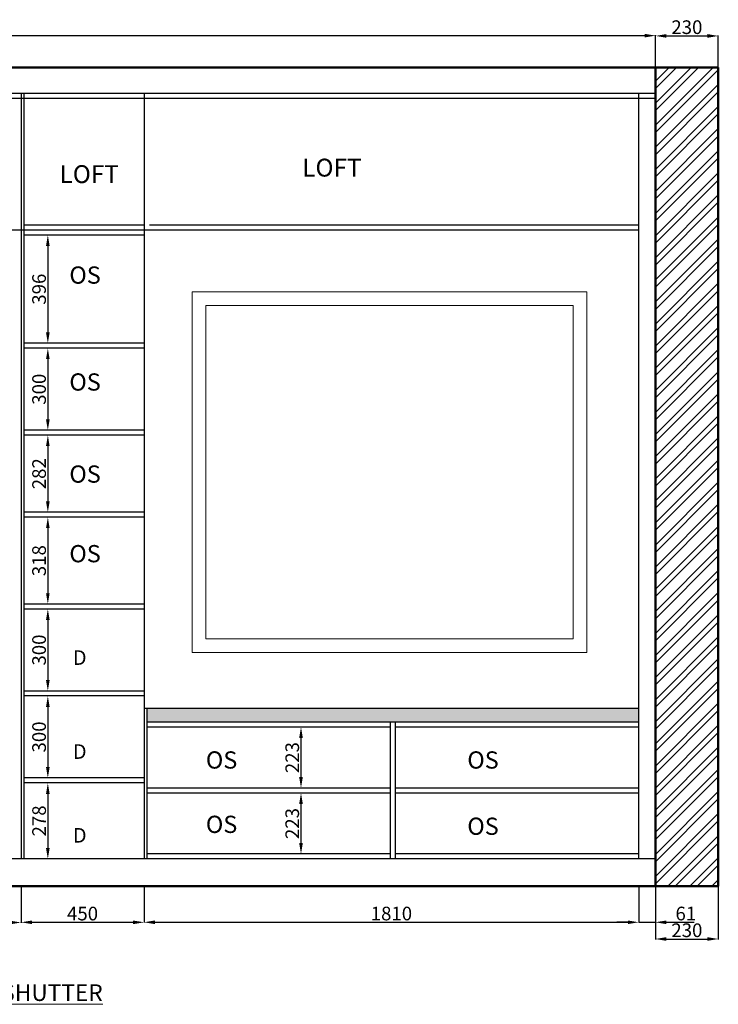
# Model space of a CAD drawing. Units: millimetres. Extents: x -513 to 5600, y -432 to 3172.
# Tile 2 of 2: x 3044 to 5600, y -432 to 3170. Entities that reach past the tile are written whole.
import ezdxf

# ---------------------------------------------------------------- set-up
doc = ezdxf.new("R2010")
doc.units = ezdxf.units.MM
for name, color, linetype, lineweight in [('A-ANNO-DIMS', 2, 'Continuous', 18), ('A-ANNO-TEXT', 7, 'Continuous', 18), ('A-ELEV-PATT', 8, 'Continuous', 13), ('A-FURN', 3, 'Continuous', 25), ('A-GLAZ', 4, 'Continuous', 18), ('A-WALL', 7, 'Continuous', 50), ('A-WALL-PATT', 8, 'Continuous', 13)]:
    doc.layers.add(name, color=color, linetype=linetype, lineweight=lineweight)
doc.styles.get("Standard").update_dxf_attribs({"font": 'arial.ttf'})
doc.dimstyles.new('ISO-25', dxfattribs={"dimtxt": 50, "dimasz": 40, "dimexe": 1.25, "dimexo": 0.625, "dimgap": 0, "dimtad": 1, "dimtxsty": 'Standard', "dimcen": 2.5, "dimclrt": 6, "dimadec": 0, "dimazin": 0, "dimtfac": 1, "dimtmove": 0, "dimatfit": 3, "dimfxl": 1, "dimarcsym": 0})

# ---------------------------------------------------------------- blocks, each defined once
blk = doc.blocks.new('*D11')
at = {"layer": 'A-ANNO-DIMS', "color": 0, "lineweight": -2, "transparency": 16777216}
for p, q in [((2129, -0.6), (2129, -133.8)), ((3049, -0.6), (3049, -133.8)), ((2169, -132.6), (3009, -132.6))]:
    blk.add_line(p, q, dxfattribs=at)
at = {"layer": 'A-ANNO-DIMS', "color": 0, "transparency": 16777216}
for points in [[(2169, -125.9), (2169, -139.2), (2129, -132.6)], [(3009, -125.9), (3009, -139.2), (3049, -132.6)]]:
    blk.add_solid(points, dxfattribs=at)
at = {"layer": 'Defpoints', "color": 0, "transparency": 16777216}
for p in [(2129, 0), (3049, 0), (3049, -132.6)]:
    blk.add_point(p, dxfattribs=at)
at = {"layer": 'A-ANNO-DIMS', "color": 0, "transparency": 16777216, "insert": (2589, -107), "char_height": 50, "attachment_point": 5}
blk.add_mtext('920', dxfattribs=at)
blk = doc.blocks.new('*D12')
at = {"layer": 'A-ANNO-DIMS', "color": 0, "lineweight": -2, "transparency": 16777216}
for p, q in [((3049, -0.6), (3049, -133.2)), ((3499, -0.6), (3499, -133.2)), ((3089, -131.9), (3459, -131.9))]:
    blk.add_line(p, q, dxfattribs=at)
at = {"layer": 'A-ANNO-DIMS', "color": 0, "transparency": 16777216}
for points in [[(3089, -125.3), (3089, -138.6), (3049, -131.9)], [(3459, -125.3), (3459, -138.6), (3499, -131.9)]]:
    blk.add_solid(points, dxfattribs=at)
at = {"layer": 'Defpoints', "color": 0, "transparency": 16777216}
for p in [(3049, 0), (3499, 0), (3499, -131.9)]:
    blk.add_point(p, dxfattribs=at)
at = {"layer": 'A-ANNO-DIMS', "color": 0, "transparency": 16777216, "insert": (3274, -106.4), "char_height": 50, "attachment_point": 5}
blk.add_mtext('450', dxfattribs=at)
blk = doc.blocks.new('*D13')
at = {"layer": 'A-ANNO-DIMS', "color": 0, "lineweight": -2, "transparency": 16777216}
for p, q in [((3499, -0.6), (3499, -133.1)), ((5309, -0.6), (5309, -133.1)), ((3539, -131.8), (5269, -131.8))]:
    blk.add_line(p, q, dxfattribs=at)
at = {"layer": 'A-ANNO-DIMS', "color": 0, "transparency": 16777216}
for points in [[(3539, -125.2), (3539, -138.5), (3499, -131.8)], [(5269, -125.2), (5269, -138.5), (5309, -131.8)]]:
    blk.add_solid(points, dxfattribs=at)
at = {"layer": 'Defpoints', "color": 0, "transparency": 16777216}
for p in [(3499, 0), (5309, 0), (5309, -131.8)]:
    blk.add_point(p, dxfattribs=at)
at = {"layer": 'A-ANNO-DIMS', "color": 0, "transparency": 16777216, "insert": (4404, -106.3), "char_height": 50, "attachment_point": 5}
blk.add_mtext('1810', dxfattribs=at)
blk = doc.blocks.new('*D14')
at = {"layer": 'A-ANNO-DIMS', "color": 0, "lineweight": -2, "transparency": 16777216}
for p, q in [((5309, -0.6), (5309, -133.1)), ((5370, -0.6), (5370, -133.1)), ((5269, -131.8), (5229, -131.8)), ((5309, -131.8), (5370, -131.8)), ((5410, -131.8), (5512.2, -131.8))]:
    blk.add_line(p, q, dxfattribs=at)
at = {"layer": 'A-ANNO-DIMS', "color": 0, "transparency": 16777216}
for points in [[(5269, -125.2), (5269, -138.5), (5309, -131.8)], [(5410, -125.2), (5410, -138.5), (5370, -131.8)]]:
    blk.add_solid(points, dxfattribs=at)
at = {"layer": 'Defpoints', "color": 0, "transparency": 16777216}
for p in [(5309, 0), (5370, 0), (5370, -131.8)]:
    blk.add_point(p, dxfattribs=at)
at = {"layer": 'A-ANNO-DIMS', "color": 0, "transparency": 16777216, "insert": (5481.1, -106.3), "char_height": 50, "attachment_point": 5}
blk.add_mtext('61', dxfattribs=at)
blk = doc.blocks.new('*D15')
at = {"layer": 'A-ANNO-DIMS', "color": 0, "lineweight": -2, "transparency": 16777216}
for p, q in [((5370, -0.6), (5370, -194.2)), ((5600, -0.6), (5600, -194.2)), ((5410, -193), (5560, -193))]:
    blk.add_line(p, q, dxfattribs=at)
at = {"layer": 'A-ANNO-DIMS', "color": 0, "transparency": 16777216}
for points in [[(5410, -186.3), (5410, -199.6), (5370, -193)], [(5560, -186.3), (5560, -199.6), (5600, -193)]]:
    blk.add_solid(points, dxfattribs=at)
at = {"layer": 'Defpoints', "color": 0, "transparency": 16777216}
for p in [(5370, 0), (5600, 0), (5600, -193)]:
    blk.add_point(p, dxfattribs=at)
at = {"layer": 'A-ANNO-DIMS', "color": 0, "transparency": 16777216, "insert": (5485, -167.4), "char_height": 50, "attachment_point": 5}
blk.add_mtext('230', dxfattribs=at)
blk = doc.blocks.new('*D30')
at = {"layer": 'A-ANNO-DIMS', "color": 0, "lineweight": -2, "transparency": 16777216}
for p, q in [((3147.6, 2382), (3148.2, 2382)), ((3147, 2342), (3147, 2026)), ((3147.6, 1986), (3148.2, 1986))]:
    blk.add_line(p, q, dxfattribs=at)
at = {"layer": 'A-ANNO-DIMS', "color": 0, "transparency": 16777216}
for points in [[(3140.3, 2342), (3153.6, 2342), (3147, 2382)], [(3140.3, 2026), (3153.6, 2026), (3147, 1986)]]:
    blk.add_solid(points, dxfattribs=at)
at = {"layer": 'Defpoints', "color": 0, "transparency": 16777216}
for p in [(3147, 2382), (3147, 1986), (3147, 1986)]:
    blk.add_point(p, dxfattribs=at)
at = {"layer": 'A-ANNO-DIMS', "color": 0, "transparency": 16777216, "insert": (3121.4, 2184), "char_height": 50, "attachment_point": 5, "rotation": 90}
blk.add_mtext('396', dxfattribs=at)
blk = doc.blocks.new('*D31')
at = {"layer": 'A-ANNO-DIMS', "color": 0, "lineweight": -2, "transparency": 16777216}
for p, q in [((3147.6, 1968), (3148.2, 1968)), ((3147, 1928), (3147, 1708)), ((3147.6, 1668), (3148.2, 1668))]:
    blk.add_line(p, q, dxfattribs=at)
at = {"layer": 'A-ANNO-DIMS', "color": 0, "transparency": 16777216}
for points in [[(3140.3, 1928), (3153.6, 1928), (3147, 1968)], [(3140.3, 1708), (3153.6, 1708), (3147, 1668)]]:
    blk.add_solid(points, dxfattribs=at)
at = {"layer": 'Defpoints', "color": 0, "transparency": 16777216}
for p in [(3147, 1968), (3147, 1668), (3147, 1668)]:
    blk.add_point(p, dxfattribs=at)
at = {"layer": 'A-ANNO-DIMS', "color": 0, "transparency": 16777216, "insert": (3121.4, 1818), "char_height": 50, "attachment_point": 5, "rotation": 90}
blk.add_mtext('300', dxfattribs=at)
blk = doc.blocks.new('*D32')
at = {"layer": 'A-ANNO-DIMS', "color": 0, "lineweight": -2, "transparency": 16777216}
for p, q in [((3147.6, 1650), (3148.2, 1650)), ((3147, 1610), (3147, 1408)), ((3147.6, 1368), (3148.2, 1368))]:
    blk.add_line(p, q, dxfattribs=at)
at = {"layer": 'A-ANNO-DIMS', "color": 0, "transparency": 16777216}
for points in [[(3140.3, 1610), (3153.6, 1610), (3147, 1650)], [(3140.3, 1408), (3153.6, 1408), (3147, 1368)]]:
    blk.add_solid(points, dxfattribs=at)
at = {"layer": 'Defpoints', "color": 0, "transparency": 16777216}
for p in [(3147, 1650), (3147, 1368), (3147, 1368)]:
    blk.add_point(p, dxfattribs=at)
at = {"layer": 'A-ANNO-DIMS', "color": 0, "transparency": 16777216, "insert": (3121.5, 1509), "char_height": 50, "attachment_point": 5, "rotation": 90}
blk.add_mtext('282', dxfattribs=at)
blk = doc.blocks.new('*D33')
at = {"layer": 'A-ANNO-DIMS', "color": 0, "lineweight": -2, "transparency": 16777216}
for p, q in [((3147.6, 1350), (3148.2, 1350)), ((3147, 1310), (3147, 1072)), ((3147.6, 1032), (3148.2, 1032))]:
    blk.add_line(p, q, dxfattribs=at)
at = {"layer": 'A-ANNO-DIMS', "color": 0, "transparency": 16777216}
for points in [[(3140.3, 1310), (3153.6, 1310), (3147, 1350)], [(3140.3, 1072), (3153.6, 1072), (3147, 1032)]]:
    blk.add_solid(points, dxfattribs=at)
at = {"layer": 'Defpoints', "color": 0, "transparency": 16777216}
for p in [(3147, 1350), (3147, 1032), (3147, 1032)]:
    blk.add_point(p, dxfattribs=at)
at = {"layer": 'A-ANNO-DIMS', "color": 0, "transparency": 16777216, "insert": (3121.4, 1191), "char_height": 50, "attachment_point": 5, "rotation": 90}
blk.add_mtext('318', dxfattribs=at)
blk = doc.blocks.new('*D34')
at = {"layer": 'A-ANNO-DIMS', "color": 0, "lineweight": -2, "transparency": 16777216}
for p, q in [((3147.6, 1014), (3148.2, 1014)), ((3147, 974), (3147, 754)), ((3147.6, 714), (3148.2, 714))]:
    blk.add_line(p, q, dxfattribs=at)
at = {"layer": 'A-ANNO-DIMS', "color": 0, "transparency": 16777216}
for points in [[(3140.3, 974), (3153.6, 974), (3147, 1014)], [(3140.3, 754), (3153.6, 754), (3147, 714)]]:
    blk.add_solid(points, dxfattribs=at)
at = {"layer": 'Defpoints', "color": 0, "transparency": 16777216}
for p in [(3147, 1014), (3147, 714), (3147, 714)]:
    blk.add_point(p, dxfattribs=at)
at = {"layer": 'A-ANNO-DIMS', "color": 0, "transparency": 16777216, "insert": (3121.4, 864), "char_height": 50, "attachment_point": 5, "rotation": 90}
blk.add_mtext('300', dxfattribs=at)
blk = doc.blocks.new('*D35')
at = {"layer": 'A-ANNO-DIMS', "color": 0, "lineweight": -2, "transparency": 16777216}
for p, q in [((3147.6, 696), (3148.2, 696)), ((3147, 656), (3147, 436)), ((3147.6, 396), (3148.2, 396))]:
    blk.add_line(p, q, dxfattribs=at)
at = {"layer": 'A-ANNO-DIMS', "color": 0, "transparency": 16777216}
for points in [[(3140.3, 656), (3153.6, 656), (3147, 696)], [(3140.3, 436), (3153.6, 436), (3147, 396)]]:
    blk.add_solid(points, dxfattribs=at)
at = {"layer": 'Defpoints', "color": 0, "transparency": 16777216}
for p in [(3147, 696), (3147, 396), (3147, 396)]:
    blk.add_point(p, dxfattribs=at)
at = {"layer": 'A-ANNO-DIMS', "color": 0, "transparency": 16777216, "insert": (3121.4, 546), "char_height": 50, "attachment_point": 5, "rotation": 90}
blk.add_mtext('300', dxfattribs=at)
blk = doc.blocks.new('*D36')
at = {"layer": 'A-ANNO-DIMS', "color": 0, "lineweight": -2, "transparency": 16777216}
for p, q in [((3147.6, 378), (3148.2, 378)), ((3147, 338), (3147, 140)), ((3147.6, 100), (3148.2, 100))]:
    blk.add_line(p, q, dxfattribs=at)
at = {"layer": 'A-ANNO-DIMS', "color": 0, "transparency": 16777216}
for points in [[(3140.3, 338), (3153.6, 338), (3147, 378)], [(3140.3, 140), (3153.6, 140), (3147, 100)]]:
    blk.add_solid(points, dxfattribs=at)
at = {"layer": 'Defpoints', "color": 0, "transparency": 16777216}
for p in [(3147, 378), (3147, 100), (3147, 100)]:
    blk.add_point(p, dxfattribs=at)
at = {"layer": 'A-ANNO-DIMS', "color": 0, "transparency": 16777216, "insert": (3121.5, 239), "char_height": 50, "attachment_point": 5, "rotation": 90}
blk.add_mtext('278', dxfattribs=at)
blk = doc.blocks.new('*D37')
at = {"layer": 'A-ANNO-DIMS', "color": 0, "lineweight": -2, "transparency": 16777216}
for p, q in [((4073.8, 582), (4074.4, 582)), ((4073.2, 542), (4073.2, 399)), ((4073.8, 359), (4074.4, 359))]:
    blk.add_line(p, q, dxfattribs=at)
at = {"layer": 'A-ANNO-DIMS', "color": 0, "transparency": 16777216}
for points in [[(4066.5, 542), (4079.9, 542), (4073.2, 582)], [(4066.5, 399), (4079.9, 399), (4073.2, 359)]]:
    blk.add_solid(points, dxfattribs=at)
at = {"layer": 'Defpoints', "color": 0, "transparency": 16777216}
for p in [(4073.2, 582), (4073.2, 359), (4073.2, 359)]:
    blk.add_point(p, dxfattribs=at)
at = {"layer": 'A-ANNO-DIMS', "color": 0, "transparency": 16777216, "insert": (4047.6, 470.5), "char_height": 50, "attachment_point": 5, "rotation": 90}
blk.add_mtext('223', dxfattribs=at)
blk = doc.blocks.new('*D38')
at = {"layer": 'A-ANNO-DIMS', "color": 0, "lineweight": -2, "transparency": 16777216}
for p, q in [((4073.8, 341), (4074.4, 341)), ((4073.2, 301), (4073.2, 158)), ((4073.8, 118), (4074.4, 118))]:
    blk.add_line(p, q, dxfattribs=at)
at = {"layer": 'A-ANNO-DIMS', "color": 0, "transparency": 16777216}
for points in [[(4066.5, 301), (4079.9, 301), (4073.2, 341)], [(4066.5, 158), (4079.9, 158), (4073.2, 118)]]:
    blk.add_solid(points, dxfattribs=at)
at = {"layer": 'Defpoints', "color": 0, "transparency": 16777216}
for p in [(4073.2, 341), (4073.2, 118), (4073.2, 118)]:
    blk.add_point(p, dxfattribs=at)
at = {"layer": 'A-ANNO-DIMS', "color": 0, "transparency": 16777216, "insert": (4047.6, 229.5), "char_height": 50, "attachment_point": 5, "rotation": 90}
blk.add_mtext('223', dxfattribs=at)
blk = doc.blocks.new('*D40')
at = {"layer": 'A-ANNO-DIMS', "color": 0, "lineweight": -2, "transparency": 16777216}
for p, q in [((230, 2995.6), (230, 3112.7)), ((270, 3111.4), (5330, 3111.4)), ((5370, 2995.6), (5370, 3112.7))]:
    blk.add_line(p, q, dxfattribs=at)
at = {"layer": 'A-ANNO-DIMS', "color": 0, "transparency": 16777216}
for points in [[(270, 3118.1), (270, 3104.8), (230, 3111.4)], [(5330, 3118.1), (5330, 3104.8), (5370, 3111.4)]]:
    blk.add_solid(points, dxfattribs=at)
at = {"layer": 'Defpoints', "color": 0, "transparency": 16777216}
for p in [(5370, 3111.4), (230, 2995), (5370, 2995)]:
    blk.add_point(p, dxfattribs=at)
at = {"layer": 'A-ANNO-DIMS', "color": 0, "transparency": 16777216, "insert": (2800, 3136.9), "char_height": 50, "attachment_point": 5}
blk.add_mtext('5140', dxfattribs=at)
blk = doc.blocks.new('*D41')
at = {"layer": 'A-ANNO-DIMS', "color": 0, "lineweight": -2, "transparency": 16777216}
for p, q in [((5370, 2995.6), (5370, 3111.6)), ((5410, 3110.4), (5560, 3110.4)), ((5600, 2995.6), (5600, 3111.6))]:
    blk.add_line(p, q, dxfattribs=at)
at = {"layer": 'A-ANNO-DIMS', "color": 0, "transparency": 16777216}
for points in [[(5410, 3117.1), (5410, 3103.7), (5370, 3110.4)], [(5560, 3117.1), (5560, 3103.7), (5600, 3110.4)]]:
    blk.add_solid(points, dxfattribs=at)
at = {"layer": 'Defpoints', "color": 0, "transparency": 16777216}
for p in [(5600, 3110.4), (5370, 2995), (5600, 2995)]:
    blk.add_point(p, dxfattribs=at)
at = {"layer": 'A-ANNO-DIMS', "color": 0, "transparency": 16777216, "insert": (5485, 3135.9), "char_height": 50, "attachment_point": 5}
blk.add_mtext('230', dxfattribs=at)

msp = doc.modelspace()

# ---------------------------------------------------------------- hatches: boundary and pattern name
at = {"layer": 'A-ELEV-PATT'}
h = msp.add_hatch(color=256, dxfattribs=at)
h.dxf.hatch_style = 1
h.paths.add_polyline_path([(5309, 650), (3509, 650), (3509, 600), (5309, 600)])
at = {"layer": 'A-WALL-PATT'}
h = msp.add_hatch(dxfattribs=at)
h.set_pattern_fill('ANSI32', color=256, scale=6)
h.paths.add_polyline_path([(5600, 2995), (5370, 2995), (5370, 0), (5600, 0)])

# ---------------------------------------------------------------- linework, layer by layer
at = {"layer": 'A-FURN'}
for p, q in [((5370, 2900), (300, 2900)), ((5370, 2882), (300, 2882)), ((3049, 2900), (3049, 100)), ((3059, 2900), (3059, 100)), ((3499, 2900), (3499, 100)), ((5309, 100), (5309, 2900)), ((3499, 2418), (3059, 2418)), ((5309, 2418), (3519, 2418)), ((5309, 2400), (300, 2400)), ((3499, 2382), (3059, 2382)), ((3499, 1986), (3059, 1986)), ((3499, 1968), (3059, 1968)), ((3499, 1668), (3059, 1668)), ((3499, 1650), (3059, 1650)), ((3499, 1368), (3059, 1368)), ((3499, 1350), (3059, 1350)), ((3499, 1032), (3059, 1032)), ((3499, 1014), (3059, 1014)), ((3499, 714), (3059, 714)), ((3499, 696), (3059, 696)), ((5309, 650), (3499, 650)), ((3509, 650), (3509, 100)), ((5309, 600), (3509, 600)), ((4400, 582), (3509, 582)), ((4400, 600), (4400, 100)), ((4418, 600), (4418, 100)), ((5309, 582), (4418, 582)), ((3499, 396), (3059, 396)), ((3499, 378), (3059, 378)), ((4400, 359), (3509, 359)), ((4400, 341), (3509, 341)), ((5309, 359), (4418, 359)), ((5309, 341), (4418, 341)), ((4400, 118), (3509, 118)), ((5309, 118), (4418, 118)), ((5370, 100), (230, 100))]:
    msp.add_line(p, q, dxfattribs=at)
at = {"layer": 'A-GLAZ'}
for points in [[(3675.577, 2173.778), (5118.738, 2173.778), (5118.738, 854.679), (3675.577, 854.679)], [(3725.577, 2123.778), (5068.738, 2123.778), (5068.738, 904.679), (3725.577, 904.679)]]:
    msp.add_lwpolyline(points, close=True, dxfattribs=at)
at = {"layer": 'A-WALL'}
for p, q in [((5600, 2995), (0, 2995)), ((5370, 0), (5370, 2995)), ((5600, 0), (5600, 2995)), ((0, 0), (5600, 0))]:
    msp.add_line(p, q, dxfattribs=at)

# ---------------------------------------------------------------- texts
at = {"layer": 'A-ANNO-TEXT', "char_height": 65.3441, "width": 459.1587, "attachment_point": 1}
for insert in [(3189.853, 2637.513), (4077.748, 2661.225)]:
    msp.add_mtext('{LOFT}', dxfattribs=dict(at, insert=insert))
at = {"layer": 'A-ANNO-TEXT', "attachment_point": 1}
for s, width, gutter_width, insert, char_height in [('{OS}', 5219.99715, 314.97, (3225.688, 2267.126), 62.994), ('{OS}', 5219.99715, 314.97, (3225.688, 1875.996), 62.994), ('{OS}', 5219.99715, 314.97, (3225.688, 1539.189), 62.994), ('{OS}', 5219.99715, 314.97, (3225.688, 1248.014), 62.994), ('{D}', 3812.92858, 267.268, (3238.69, 863.06), 53.4537), ('{D}', 3812.92858, 267.268, (3238.684, 519.394), 53.4537), ('{OS}', 5219.99715, 314.97, (3725.194, 493.384), 62.994), ('{OS}', 5219.99715, 314.97, (4681.687, 493.384), 62.994), ('{OS}', 5219.99715, 314.97, (3725.194, 257.92), 62.994), ('{OS}', 5219.99715, 314.97, (4681.687, 250.995), 62.994), ('{D}', 3812.92858, 267.268, (3238.684, 213.008), 53.4537), ('{\\LELEVATION WITHOUT SHUTTER}', 10157.59804, 304.543, (2123.311, -358.773), 60.90856)]:
    msp.add_mtext_dynamic_manual_height_columns(s, width=width, gutter_width=gutter_width, heights=[0], dxfattribs=dict(at, insert=insert, char_height=char_height))

# ---------------------------------------------------------------- dimensions: what is measured, and where the dimension line sits
at = {"layer": 'A-ANNO-DIMS'}
for base, p1, p2, picture, middle in [((5370, 3111.419), (230, 2995), (5370, 2995), '*D40', (2800, 3136.948)), ((5600, 3110.384), (5370, 2995), (5600, 2995), '*D41', (5485, 3135.93)), ((3049, -132.558), (2129, 0), (3049, 0), '*D11', (2589, -107.029)), ((5600, -192.968), (5370, 0), (5600, 0), '*D15', (5485, -167.423)), ((3499, -131.945), (3049, 0), (3499, 0), '*D12', (3274, -106.416)), ((5370, -131.84), (5309, 0), (5370, 0), '*D14', (5481.122, -106.311))]:
    dim = msp.add_linear_dim(base=base, p1=p1, p2=p2, dimstyle='ISO-25', override={"dimclrd": 0, "dimclre": 0, "dimclrt": 0}, dxfattribs=at)
    dim.commit()
    dim.dimension.update_dxf_attribs({"geometry": picture, "text_midpoint": middle})
for base, p1, p2, picture, middle in [((3146.982, 1986), (3146.982, 2382), (3146.982, 1986), '*D30', (3121.437, 2184)), ((3146.982, 1668), (3146.982, 1968), (3146.982, 1668), '*D31', (3121.437, 1818)), ((3146.982, 1368), (3146.982, 1650), (3146.982, 1368), '*D32', (3121.454, 1509)), ((3146.982, 1032), (3146.982, 1350), (3146.982, 1032), '*D33', (3121.437, 1191)), ((3146.982, 714), (3146.982, 1014), (3146.982, 714), '*D34', (3121.437, 864)), ((3146.982, 396), (3146.982, 696), (3146.982, 396), '*D35', (3121.437, 546)), ((4073.189, 359), (4073.189, 582), (4073.189, 359), '*D37', (4047.643, 470.5)), ((3146.982, 100), (3146.982, 378), (3146.982, 100), '*D36', (3121.454, 239)), ((4073.189, 118), (4073.189, 341), (4073.189, 118), '*D38', (4047.643, 229.5))]:
    dim = msp.add_linear_dim(base=base, p1=p1, p2=p2, angle=90, dimstyle='ISO-25', override={"dimclrd": 0, "dimclre": 0, "dimclrt": 0}, dxfattribs=at)
    dim.commit()
    dim.dimension.update_dxf_attribs({"geometry": picture, "text_midpoint": middle})
dim = msp.add_aligned_dim(p1=(3499, 0), p2=(5309, 0), distance=-131.84, dimstyle='ISO-25', override={"dimclrd": 0, "dimclre": 0, "dimclrt": 0}, dxfattribs=at)
dim.commit()
dim.dimension.update_dxf_attribs({"geometry": '*D13', "text_midpoint": (4404, -106.311)})

doc.saveas('drawing.dxf')
